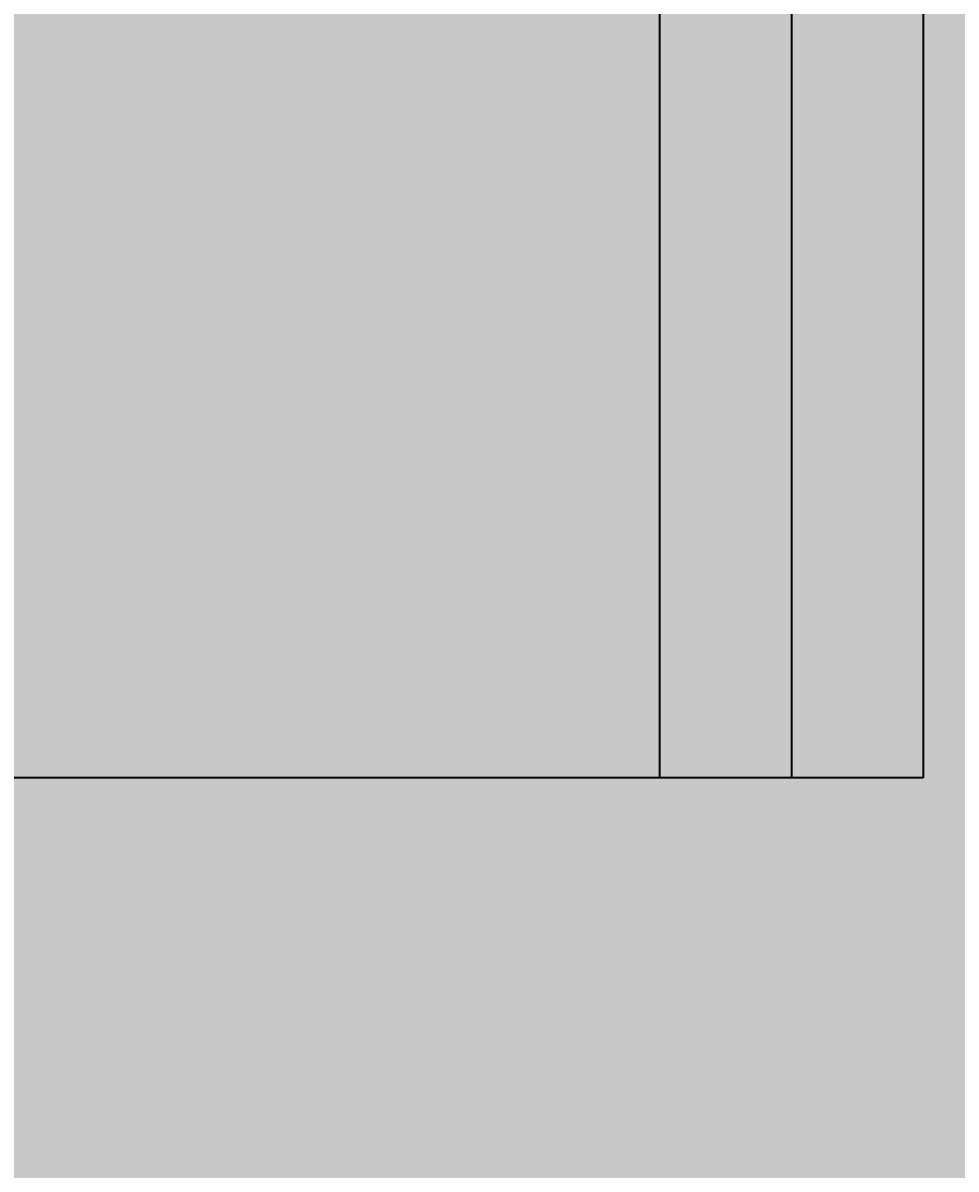
# Model space of a CAD drawing. Units: inches. Extents: x -1 to 292, y -3 to 199.
# Tile 24 of 52: x 127 to 148, y 42 to 68. Entities that reach past the tile are written whole.
import ezdxf

# ---------------------------------------------------------------- set-up
doc = ezdxf.new("R2010")
doc.units = ezdxf.units.IN
doc.header["$MEASUREMENT"] = 0
for name, color, linetype, lineweight in [('M-DIMS', 2, 'Continuous', 18), ('M-EQPM', 7, 'Continuous', 35), ('M-PATT', 8, 'Continuous', 13)]:
    doc.layers.add(name, color=color, linetype=linetype, lineweight=lineweight)
doc.styles.get("Standard").update_dxf_attribs({"font": 'arial.ttf'})
doc.dimstyles.get("Standard").update_dxf_attribs({"dimtxt": 0.18, "dimasz": 0.18, "dimexe": 0.18, "dimexo": 0.0625, "dimgap": 0.09, "dimtad": 0, "dimtih": 1, "dimtoh": 1, "dimdec": 4, "dimzin": 0, "dimdsep": 46, "dimtxsty": 'Standard', "dimcen": 0.09, "dimadec": 0, "dimazin": 0, "dimtfac": 1, "dimtdec": 4, "dimtofl": 0, "dimtmove": 0, "dimatfit": 3, "dimfxl": 1, "dimtolj": 1, "dimtzin": 0, "dimarcsym": 0})

# ---------------------------------------------------------------- blocks, each defined once
blk = doc.blocks.new('*D7')
at = {"layer": 'Defpoints', "color": 0, "transparency": 16777216}
for p in [(21.861, 54.582), (205.115, 54.582), (21.861, 39.982)]:
    blk.add_point(p, dxfattribs=at)
at = {"layer": 'M-DIMS', "color": 0, "lineweight": -2, "transparency": 16777216}
for p, q in [((21.861, 54.52), (21.861, 39.802)), ((205.115, 54.52), (205.115, 39.802)), ((22.041, 39.982), (113.033, 39.982)), ((204.935, 39.982), (113.944, 39.982))]:
    blk.add_line(p, q, dxfattribs=at)
at = {"layer": 'M-DIMS', "color": 0, "transparency": 16777216}
for points in [[(22.041, 40.012), (22.041, 39.952), (21.861, 39.982)], [(204.935, 40.012), (204.935, 39.952), (205.115, 39.982)]]:
    blk.add_solid(points, dxfattribs=at)
at = {"layer": 'M-DIMS', "color": 0, "transparency": 16777216, "insert": (113.488, 39.982), "char_height": 0.18, "attachment_point": 5}
blk.add_mtext('\\A1;183.25', dxfattribs=at)

msp = doc.modelspace()

# ---------------------------------------------------------------- hatches: boundary and pattern name
at = {"layer": 'M-PATT'}
h = msp.add_hatch(color=256, dxfattribs=at)
h.set_gradient(color1=(237, 31, 36), color2=(242, 113, 114), tint=1, name='CYLINDER')
h.paths.add_polyline_path([(106.0735, 105.9941), (106.0735, 106.9941), (108.0603, 106.9941), (107.8488, 107.6501), (57.8007, 107.6501, 0.4142136), (49.9241, 99.7735), (52.3176, 101.3278), (55.0097, 99.7735), (57.4032, 101.3278), (60.0953, 99.7735), (62.4888, 101.3278), (65.1809, 99.7735), (67.5744, 101.3278), (70.2665, 99.7735), (72.66, 101.3278), (75.3521, 99.7735), (77.7456, 101.3278), (80.4377, 99.7735), (82.8312, 101.3278), (85.5233, 99.7735), (87.9168, 101.3278), (90.6089, 99.7735), (93.0024, 101.3278), (95.6945, 99.7735), (98.088, 101.3278), (100.7801, 99.7735), (103.1736, 101.3278), (105.8657, 99.7735), (108.2592, 101.3278), (110.9513, 99.7735), (113.3448, 101.3278), (116.0369, 99.7735), (118.4304, 101.3278), (121.1225, 99.7735), (123.516, 101.3278), (126.2082, 99.7735), (128.6016, 101.3278), (131.2938, 99.7735), (133.6872, 101.3278), (136.3794, 99.7735), (138.7728, 101.3278), (141.465, 99.7735), (143.8584, 101.3278), (146.5506, 99.7735), (148.944, 101.3278), (151.6362, 99.7735), (154.0296, 101.3278), (156.7218, 99.7735), (159.1152, 101.3278), (160.6222, 100.4578), (160.6222, 107.6501), (115.4883, 107.6501), (115.4883, 106.9941), (120.9032, 106.9941), (120.9032, 105.9941), (120.9032, 103.3981), (106.0735, 103.3981)])
h.paths.add_polyline_path([(169.176, 107.6501), (162.1623, 107.6501), (162.1623, 100.004), (164.2008, 101.3278), (166.893, 99.7735), (169.2864, 101.3278), (171.9786, 99.7735), (174.372, 101.3278), (177.0526, 99.7802, 0.4139642)])
h.paths.add_polyline_path([(111.4883, 107.6501), (107.8488, 107.6501), (108.0603, 106.9941), (111.4883, 106.9941)], flags=17)
h.paths.add_polyline_path([(61.6788, 91.897), (57.8007, 91.897, -0.1099266), (54.4604, 92.6403), (43.2011, 92.6403), (23.9502, 84.4688), (23.9502, 58.376), (43.2011, 47.2615), (50.9409, 47.2615, -0.2705926), (57.8007, 51.2672), (61.6788, 51.2672)])
h.paths.add_polyline_path([(73.6788, 91.897), (70.6788, 91.897), (70.6788, 51.2672), (73.6788, 51.2672)])
h.paths.add_polyline_path([(79.6788, 91.897), (76.6788, 91.897), (76.6788, 51.2672), (79.6788, 51.2672)])
h.paths.add_polyline_path([(67.6788, 91.897), (64.6788, 91.897), (64.6788, 51.2672), (67.6788, 51.2672)])
h.paths.add_polyline_path([(101.6788, 91.897), (82.6788, 91.897), (82.6788, 51.2672), (101.6788, 51.2672)])
h.paths.add_polyline_path([(107.6788, 91.897), (104.6788, 91.897), (104.6788, 51.2672), (107.6788, 51.2672)])
h.paths.add_polyline_path([(113.6788, 91.897), (110.6788, 91.897), (110.6788, 51.2672), (113.6788, 51.2672)])
h.paths.add_polyline_path([(119.6788, 91.897), (116.6788, 91.897), (116.6788, 51.2672), (119.6788, 51.2672)])
h.paths.add_polyline_path([(141.6788, 91.897), (122.6788, 91.897), (122.6788, 51.2672), (141.6788, 51.2672)])
h.paths.add_polyline_path([(147.6788, 91.897), (144.6788, 91.897), (144.6788, 51.2672), (147.6788, 51.2672)])
h.paths.add_polyline_path([(153.6788, 91.897), (150.6788, 91.897), (150.6788, 51.2672), (153.6788, 51.2672)])
h.paths.add_polyline_path([(159.6788, 91.897), (156.6788, 91.897), (156.6788, 51.2672), (159.6788, 51.2672)])
h.paths.add_polyline_path([(179.5897, 92.6403), (172.5163, 92.6403, -0.1099266), (169.176, 91.897), (162.6788, 91.897), (162.6788, 51.2672), (169.176, 51.2672, -0.2705926), (176.0358, 47.2615), (179.5897, 47.2615)])
h.paths.add_polyline_path([(203.0265, 84.4688), (183.7755, 92.6403), (181.5897, 92.6403), (181.5897, 47.2615), (183.7755, 47.2615), (203.0265, 58.376)])
h.paths.add_polyline_path([(184.4188, 61.52), (200.7224, 61.52), (200.7224, 77.7532), (184.4188, 77.7532)], flags=24)
h = msp.add_hatch(color=256, dxfattribs=at)
h.set_gradient(color1=(0, 255, 255), color2=(0, 255, 255), tint=1)
h.paths.add_polyline_path([(75.3521, 99.7735), (72.66, 101.3278), (70.2665, 99.7735), (67.5744, 101.3278), (65.1809, 99.7735), (62.4888, 101.3278), (60.0953, 99.7735), (57.4032, 101.3278), (55.0097, 99.7735), (52.3176, 101.3278), (49.9241, 99.7735, 0.4142136), (57.8007, 91.897), (61.6788, 91.897), (61.6788, 51.2672), (57.8007, 51.2672, 0.8088808), (54.5813, 36.2021), (65.0947, 51.2672), (64.6788, 51.2672), (64.6788, 91.897), (67.6788, 91.897), (67.6788, 51.2672), (65.0947, 51.2672), (54.5813, 36.2021, 0.1056561), (57.8007, 35.5141), (169.176, 35.5141, 1), (169.176, 51.2672), (162.6788, 51.2672), (162.6788, 91.897), (169.176, 91.897, 0.4144629), (177.0526, 99.7802), (174.372, 101.3278), (171.9786, 99.7735), (169.2864, 101.3278), (166.893, 99.7735), (164.2008, 101.3278), (162.1623, 100.004), (162.1623, 96.1027), (160.6222, 96.1027), (160.6222, 100.4578), (159.1152, 101.3278), (156.7218, 99.7735), (154.0296, 101.3278), (151.6362, 99.7735), (148.944, 101.3278), (146.5506, 99.7735), (143.8584, 101.3278), (141.465, 99.7735), (138.7728, 101.3278), (136.3794, 99.7735), (133.6872, 101.3278), (131.2938, 99.7735), (128.6016, 101.3278), (126.2082, 99.7735), (123.516, 101.3278), (121.1225, 99.7735), (118.4304, 101.3278), (116.0369, 99.7735), (113.3448, 101.3278), (110.9513, 99.7735), (108.2592, 101.3278), (105.8657, 99.7735), (103.1736, 101.3278), (100.7801, 99.7735), (98.088, 101.3278), (95.6945, 99.7735), (93.0024, 101.3278), (90.6089, 99.7735), (87.9168, 101.3278), (85.5233, 99.7735), (82.8312, 101.3278), (80.4377, 99.7735), (77.7456, 101.3278)])
h.paths.add_polyline_path([(79.6788, 91.897), (79.6788, 51.2672), (76.6788, 51.2672), (76.6788, 91.897)], flags=16)
h.paths.add_polyline_path([(73.6788, 91.897), (73.6788, 51.2672), (70.6788, 51.2672), (70.6788, 91.897)], flags=16)
h.paths.add_polyline_path([(82.6788, 91.897), (101.6788, 91.897), (101.6788, 51.2672), (82.6788, 51.2672)], flags=16)
h.paths.add_polyline_path([(104.6788, 91.897), (107.6788, 91.897), (107.6788, 51.2672), (104.6788, 51.2672)], flags=16)
h.paths.add_polyline_path([(110.6788, 91.897), (113.6788, 91.897), (113.6788, 51.2672), (110.6788, 51.2672)], flags=16)
h.paths.add_polyline_path([(116.6788, 91.897), (119.6788, 91.897), (119.6788, 51.2672), (116.6788, 51.2672)], flags=16)
h.paths.add_polyline_path([(122.6788, 91.897), (141.6788, 91.897), (141.6788, 51.2672), (144.6788, 51.2672), (144.6788, 91.897), (147.6788, 91.897), (147.6788, 51.2672), (122.6788, 51.2672)], flags=16)
h.paths.add_polyline_path([(150.6788, 91.897), (153.6788, 91.897), (153.6788, 51.2672), (150.6788, 51.2672)], flags=16)
h.paths.add_polyline_path([(156.6788, 91.897), (159.6788, 91.897), (159.6788, 51.2672), (156.6788, 51.2672)], flags=16)

# ---------------------------------------------------------------- linework, layer by layer
at = {"layer": 'M-EQPM'}
for p, q in [((141.6788, 91.897), (141.6788, 51.2672)), ((144.6788, 91.897), (144.6788, 51.2672)), ((147.6788, 91.897), (147.6788, 51.2672))]:
    msp.add_line(p, q, dxfattribs=at)
msp.add_lwpolyline([(147.6788, 51.2672), (122.6788, 51.2672)], dxfattribs=at)

# ---------------------------------------------------------------- dimensions: what is measured, and where the dimension line sits
at = {"layer": 'M-DIMS'}
dim = msp.add_linear_dim(base=(21.8612, 39.9821), p1=(205.1155, 54.5821), p2=(21.8612, 54.5821), angle=180, dimstyle='Standard', override={"dimdec": 2, "dimlfac": 1, "dimrnd": 0, "dimzin": 0, "dimdsep": 46, "dimlunit": 2}, dxfattribs=at)
dim.commit()
dim.dimension.update_dxf_attribs({"geometry": '*D7', "text_midpoint": (113.4883, 39.9821)})

doc.saveas('drawing.dxf')
